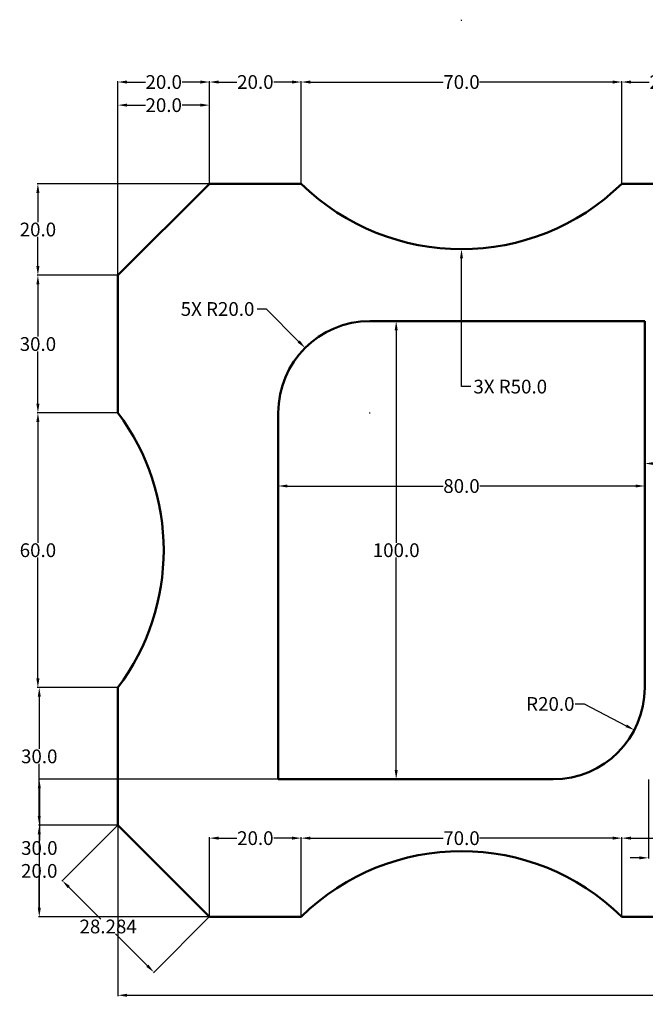
# Model space of a CAD drawing. Units: inches. Extents: x 142 to 482, y 54 to 269.
# Tile 1 of 2: x 142 to 279, y 54 to 269. Entities that reach past the tile are written whole.
import ezdxf

# ---------------------------------------------------------------- set-up
doc = ezdxf.new("R2010")
doc.units = ezdxf.units.IN
doc.header["$MEASUREMENT"] = 0
doc.layers.add('M-DIMS', color=2, linetype='Continuous', lineweight=25)
doc.layers.add('M-OUTL', color=7, linetype='Continuous', lineweight=50)
doc.styles.get("Standard").update_dxf_attribs({"font": 'arial.ttf'})
doc.dimstyles.get("Standard").update_dxf_attribs({"dimtxt": 3, "dimasz": 2, "dimexe": 0.18, "dimexo": 0.0625, "dimgap": 0.09, "dimtad": 0, "dimtih": 1, "dimtoh": 1, "dimdec": 1, "dimzin": 0, "dimdsep": 46, "dimtxsty": 'Standard', "dimcen": 0.09, "dimclrd": 1, "dimclre": 1, "dimadec": 0, "dimazin": 0, "dimtfac": 1, "dimtdec": 1, "dimtofl": 0, "dimtmove": 0, "dimatfit": 3, "dimfxl": 1, "dimtolj": 1, "dimtzin": 0, "dimarcsym": 0})

# ---------------------------------------------------------------- blocks, each defined once
blk = doc.blocks.new('*D1')
at = {"layer": 'Defpoints', "color": 0, "transparency": 16777216}
for p in [(146.28, 183.54), (163.74, 183.54), (163.74, 123.54)]:
    blk.add_point(p, dxfattribs=at)
at = {"layer": 'M-DIMS', "color": 0, "lineweight": -2, "transparency": 16777216}
for p, q in [((163.67, 183.54), (146.1, 183.54)), ((146.28, 181.54), (146.28, 155.16)), ((146.28, 125.54), (146.28, 151.92)), ((163.67, 123.54), (146.1, 123.54))]:
    blk.add_line(p, q, dxfattribs=at)
at = {"layer": 'M-DIMS', "color": 0, "transparency": 16777216}
for points in [[(145.94, 181.54), (146.61, 181.54), (146.28, 183.54)], [(145.94, 125.54), (146.61, 125.54), (146.28, 123.54)]]:
    blk.add_solid(points, dxfattribs=at)
at = {"layer": 'M-DIMS', "color": 0, "transparency": 16777216, "insert": (146.28, 153.54), "char_height": 3, "attachment_point": 5}
blk.add_mtext('\\A1;60.0', dxfattribs=at)
blk = doc.blocks.new('*D2')
at = {"layer": 'Defpoints', "color": 0, "transparency": 16777216}
for p in [(163.74, 93.54), (146.57, 73.54), (183.74, 73.54)]:
    blk.add_point(p, dxfattribs=at)
at = {"layer": 'M-DIMS', "color": 0, "lineweight": -2, "transparency": 16777216}
for p, q in [((163.67, 93.54), (146.39, 93.54)), ((146.57, 91.54), (146.57, 85.16)), ((146.57, 75.54), (146.57, 81.92)), ((183.67, 73.54), (146.39, 73.54))]:
    blk.add_line(p, q, dxfattribs=at)
at = {"layer": 'M-DIMS', "color": 0, "transparency": 16777216}
for points in [[(146.24, 91.54), (146.91, 91.54), (146.57, 93.54)], [(146.24, 75.54), (146.91, 75.54), (146.57, 73.54)]]:
    blk.add_solid(points, dxfattribs=at)
at = {"layer": 'M-DIMS', "color": 0, "transparency": 16777216, "insert": (146.57, 83.54), "char_height": 3, "attachment_point": 5}
blk.add_mtext('\\A1;20.0', dxfattribs=at)
blk = doc.blocks.new('*D3')
at = {"layer": 'Defpoints', "color": 0, "transparency": 16777216}
for p in [(146.57, 123.54), (163.74, 123.54), (163.74, 93.54)]:
    blk.add_point(p, dxfattribs=at)
at = {"layer": 'M-DIMS', "color": 0, "lineweight": -2, "transparency": 16777216}
for p, q in [((163.67, 123.54), (146.39, 123.54)), ((146.57, 121.54), (146.57, 110.16)), ((146.57, 95.54), (146.57, 106.92)), ((163.67, 93.54), (146.39, 93.54))]:
    blk.add_line(p, q, dxfattribs=at)
at = {"layer": 'M-DIMS', "color": 0, "transparency": 16777216}
for points in [[(146.24, 121.54), (146.91, 121.54), (146.57, 123.54)], [(146.24, 95.54), (146.91, 95.54), (146.57, 93.54)]]:
    blk.add_solid(points, dxfattribs=at)
at = {"layer": 'M-DIMS', "color": 0, "transparency": 16777216, "insert": (146.57, 108.54), "char_height": 3, "attachment_point": 5}
blk.add_mtext('\\A1;30.0', dxfattribs=at)
blk = doc.blocks.new('*D4')
at = {"layer": 'Defpoints', "color": 0, "transparency": 16777216}
for p in [(146.28, 213.54), (163.74, 213.54), (163.74, 183.54)]:
    blk.add_point(p, dxfattribs=at)
at = {"layer": 'M-DIMS', "color": 0, "lineweight": -2, "transparency": 16777216}
for p, q in [((163.67, 213.54), (146.1, 213.54)), ((146.28, 211.54), (146.28, 200.16)), ((146.28, 185.54), (146.28, 196.92)), ((163.67, 183.54), (146.1, 183.54))]:
    blk.add_line(p, q, dxfattribs=at)
at = {"layer": 'M-DIMS', "color": 0, "transparency": 16777216}
for points in [[(145.94, 211.54), (146.61, 211.54), (146.28, 213.54)], [(145.94, 185.54), (146.61, 185.54), (146.28, 183.54)]]:
    blk.add_solid(points, dxfattribs=at)
at = {"layer": 'M-DIMS', "color": 0, "transparency": 16777216, "insert": (146.28, 198.54), "char_height": 3, "attachment_point": 5}
blk.add_mtext('\\A1;30.0', dxfattribs=at)
blk = doc.blocks.new('*D5')
at = {"layer": 'Defpoints', "color": 0, "transparency": 16777216}
for p in [(183.74, 233.54), (146.28, 213.54), (163.74, 213.54)]:
    blk.add_point(p, dxfattribs=at)
at = {"layer": 'M-DIMS', "color": 0, "lineweight": -2, "transparency": 16777216}
for p, q in [((183.67, 233.54), (146.1, 233.54)), ((146.28, 231.54), (146.28, 225.16)), ((146.28, 215.54), (146.28, 221.92)), ((163.67, 213.54), (146.1, 213.54))]:
    blk.add_line(p, q, dxfattribs=at)
at = {"layer": 'M-DIMS', "color": 0, "transparency": 16777216}
for points in [[(145.94, 231.54), (146.61, 231.54), (146.28, 233.54)], [(145.94, 215.54), (146.61, 215.54), (146.28, 213.54)]]:
    blk.add_solid(points, dxfattribs=at)
at = {"layer": 'M-DIMS', "color": 0, "transparency": 16777216, "insert": (146.28, 223.54), "char_height": 3, "attachment_point": 5}
blk.add_mtext('\\A1;20.0', dxfattribs=at)
blk = doc.blocks.new('*D6')
at = {"layer": 'Defpoints', "color": 0, "transparency": 16777216}
for p in [(203.74, 255.73), (183.74, 233.54), (203.74, 233.54)]:
    blk.add_point(p, dxfattribs=at)
at = {"layer": 'M-DIMS', "color": 0, "lineweight": -2, "transparency": 16777216}
for p, q in [((183.74, 233.6), (183.74, 255.91)), ((203.74, 233.6), (203.74, 255.91)), ((185.74, 255.73), (189.73, 255.73)), ((201.74, 255.73), (197.74, 255.73))]:
    blk.add_line(p, q, dxfattribs=at)
at = {"layer": 'M-DIMS', "color": 0, "transparency": 16777216}
for points in [[(185.74, 256.06), (185.74, 255.39), (183.74, 255.73)], [(201.74, 256.06), (201.74, 255.39), (203.74, 255.73)]]:
    blk.add_solid(points, dxfattribs=at)
at = {"layer": 'M-DIMS', "color": 0, "transparency": 16777216, "insert": (193.74, 255.73), "char_height": 3, "attachment_point": 5}
blk.add_mtext('\\A1;20.0', dxfattribs=at)
blk = doc.blocks.new('*D7')
at = {"layer": 'Defpoints', "color": 0, "transparency": 16777216}
for p in [(163.74, 255.73), (183.74, 233.54), (163.74, 213.54)]:
    blk.add_point(p, dxfattribs=at)
at = {"layer": 'M-DIMS', "color": 0, "lineweight": -2, "transparency": 16777216}
for p, q in [((163.74, 213.6), (163.74, 255.91)), ((183.74, 233.6), (183.74, 255.91)), ((165.74, 255.73), (169.73, 255.73)), ((181.74, 255.73), (177.74, 255.73))]:
    blk.add_line(p, q, dxfattribs=at)
at = {"layer": 'M-DIMS', "color": 0, "transparency": 16777216}
for points in [[(165.74, 256.06), (165.74, 255.39), (163.74, 255.73)], [(181.74, 256.06), (181.74, 255.39), (183.74, 255.73)]]:
    blk.add_solid(points, dxfattribs=at)
at = {"layer": 'M-DIMS', "color": 0, "transparency": 16777216, "insert": (173.74, 255.73), "char_height": 3, "attachment_point": 5}
blk.add_mtext('\\A1;20.0', dxfattribs=at)
blk = doc.blocks.new('*D8')
at = {"layer": 'Defpoints', "color": 0, "transparency": 16777216}
for p in [(273.74, 255.73), (203.74, 233.54), (273.74, 233.54)]:
    blk.add_point(p, dxfattribs=at)
at = {"layer": 'M-DIMS', "color": 0, "lineweight": -2, "transparency": 16777216}
for p, q in [((203.74, 233.6), (203.74, 255.91)), ((273.74, 233.6), (273.74, 255.91)), ((205.74, 255.73), (234.77, 255.73)), ((271.74, 255.73), (242.7, 255.73))]:
    blk.add_line(p, q, dxfattribs=at)
at = {"layer": 'M-DIMS', "color": 0, "transparency": 16777216}
for points in [[(205.74, 256.06), (205.74, 255.39), (203.74, 255.73)], [(271.74, 256.06), (271.74, 255.39), (273.74, 255.73)]]:
    blk.add_solid(points, dxfattribs=at)
at = {"layer": 'M-DIMS', "color": 0, "transparency": 16777216, "insert": (238.74, 255.73), "char_height": 3, "attachment_point": 5}
blk.add_mtext('\\A1;70.0', dxfattribs=at)
blk = doc.blocks.new('*D9')
at = {"layer": 'Defpoints', "color": 0, "transparency": 16777216}
for p in [(293.74, 255.73), (273.74, 233.54), (293.74, 233.54)]:
    blk.add_point(p, dxfattribs=at)
at = {"layer": 'M-DIMS', "color": 0, "lineweight": -2, "transparency": 16777216}
for p, q in [((273.74, 233.6), (273.74, 255.91)), ((293.74, 233.6), (293.74, 255.91)), ((275.74, 255.73), (279.73, 255.73)), ((291.74, 255.73), (287.74, 255.73))]:
    blk.add_line(p, q, dxfattribs=at)
at = {"layer": 'M-DIMS', "color": 0, "transparency": 16777216}
for points in [[(275.74, 256.06), (275.74, 255.39), (273.74, 255.73)], [(291.74, 256.06), (291.74, 255.39), (293.74, 255.73)]]:
    blk.add_solid(points, dxfattribs=at)
at = {"layer": 'M-DIMS', "color": 0, "transparency": 16777216, "insert": (283.74, 255.73), "char_height": 3, "attachment_point": 5}
blk.add_mtext('\\A1;20.0', dxfattribs=at)
blk = doc.blocks.new('*D22')
at = {"layer": 'Defpoints', "color": 0, "transparency": 16777216}
for p in [(258.74, 123.54), (276.47, 114.29)]:
    blk.add_point(p, dxfattribs=at)
at = {"layer": 'M-DIMS', "color": 0, "lineweight": -2, "transparency": 16777216}
for p, q in [((263.55, 119.98), (265.55, 119.98)), ((265.55, 119.98), (274.69, 115.21))]:
    blk.add_line(p, q, dxfattribs=at)
at = {"layer": 'M-DIMS', "color": 0, "transparency": 16777216}
blk.add_solid([(274.85, 115.51), (274.54, 114.92), (276.47, 114.29)], dxfattribs=at)
at = {"layer": 'M-DIMS', "color": 0, "transparency": 16777216, "insert": (258.13, 119.98), "char_height": 3, "attachment_point": 5}
blk.add_mtext('\\A1;R20.0', dxfattribs=at)
blk = doc.blocks.new('*D23')
at = {"layer": 'Defpoints', "color": 0, "transparency": 16777216}
for p in [(248.74, 203.54), (224.48, 103.54), (228.74, 103.54)]:
    blk.add_point(p, dxfattribs=at)
at = {"layer": 'M-DIMS', "color": 0, "lineweight": -2, "transparency": 16777216}
for p, q in [((248.67, 203.54), (224.3, 203.54)), ((224.48, 201.54), (224.48, 155.16)), ((224.48, 105.54), (224.48, 151.92)), ((228.67, 103.54), (224.3, 103.54))]:
    blk.add_line(p, q, dxfattribs=at)
at = {"layer": 'M-DIMS', "color": 0, "transparency": 16777216}
for points in [[(224.15, 201.54), (224.81, 201.54), (224.48, 203.54)], [(224.15, 105.54), (224.81, 105.54), (224.48, 103.54)]]:
    blk.add_solid(points, dxfattribs=at)
at = {"layer": 'M-DIMS', "color": 0, "transparency": 16777216, "insert": (224.48, 153.54), "char_height": 3, "attachment_point": 5}
blk.add_mtext('\\A1;100.0', dxfattribs=at)
blk = doc.blocks.new('*D24')
at = {"layer": 'Defpoints', "color": 0, "transparency": 16777216}
for p in [(198.74, 183.54), (278.74, 183.54), (278.74, 167.55)]:
    blk.add_point(p, dxfattribs=at)
at = {"layer": 'M-DIMS', "color": 0, "lineweight": -2, "transparency": 16777216}
for p, q in [((198.74, 183.48), (198.74, 167.37)), ((278.74, 183.48), (278.74, 167.37)), ((200.74, 167.55), (234.75, 167.55)), ((276.74, 167.55), (242.72, 167.55))]:
    blk.add_line(p, q, dxfattribs=at)
at = {"layer": 'M-DIMS', "color": 0, "transparency": 16777216}
for points in [[(200.74, 167.88), (200.74, 167.22), (198.74, 167.55)], [(276.74, 167.88), (276.74, 167.22), (278.74, 167.55)]]:
    blk.add_solid(points, dxfattribs=at)
at = {"layer": 'M-DIMS', "color": 0, "transparency": 16777216, "insert": (238.74, 167.55), "char_height": 3, "attachment_point": 5}
blk.add_mtext('\\A1;80.0', dxfattribs=at)
blk = doc.blocks.new('*D26')
at = {"layer": 'Defpoints', "color": 0, "transparency": 16777216}
for p in [(278.74, 183.54), (313.74, 183.54), (313.74, 172.46)]:
    blk.add_point(p, dxfattribs=at)
at = {"layer": 'M-DIMS', "color": 0, "lineweight": -2, "transparency": 16777216}
for p, q in [((278.74, 183.48), (278.74, 172.28)), ((313.74, 183.48), (313.74, 172.28)), ((280.74, 172.46), (292.26, 172.46)), ((311.74, 172.46), (300.22, 172.46))]:
    blk.add_line(p, q, dxfattribs=at)
at = {"layer": 'M-DIMS', "color": 0, "transparency": 16777216}
for points in [[(280.74, 172.79), (280.74, 172.13), (278.74, 172.46)], [(311.74, 172.79), (311.74, 172.13), (313.74, 172.46)]]:
    blk.add_solid(points, dxfattribs=at)
at = {"layer": 'M-DIMS', "color": 0, "transparency": 16777216, "insert": (296.24, 172.46), "char_height": 3, "attachment_point": 5}
blk.add_mtext('\\A1;35.0', dxfattribs=at)
blk = doc.blocks.new('*D27')
at = {"layer": 'Defpoints', "color": 0, "transparency": 16777216}
for p in [(450.34, 141.94), (163.74, 93.54), (450.34, 56.39)]:
    blk.add_point(p, dxfattribs=at)
at = {"layer": 'M-DIMS', "color": 1, "lineweight": -2, "transparency": 16777216}
for p, q in [((450.34, 141.88), (450.34, 56.21)), ((163.74, 93.48), (163.74, 56.21)), ((165.74, 56.39), (301.86, 56.39)), ((448.34, 56.39), (312.21, 56.39))]:
    blk.add_line(p, q, dxfattribs=at)
at = {"layer": 'M-DIMS', "color": 1, "transparency": 16777216}
for points in [[(165.74, 56.72), (165.74, 56.06), (163.74, 56.39)], [(448.34, 56.72), (448.34, 56.06), (450.34, 56.39)]]:
    blk.add_solid(points, dxfattribs=at)
at = {"layer": 'M-DIMS', "color": 0, "transparency": 16777216, "insert": (307.04, 56.39), "char_height": 3, "attachment_point": 5}
blk.add_mtext('\\A1;286.6', dxfattribs=at)
blk = doc.blocks.new('*D29')
at = {"layer": 'Defpoints', "color": 0, "transparency": 16777216}
for p in [(198.74, 103.54), (146.59, 73.54), (183.74, 73.54)]:
    blk.add_point(p, dxfattribs=at)
at = {"layer": 'M-DIMS', "color": 1, "lineweight": -2, "transparency": 16777216}
for p, q in [((198.67, 103.54), (146.41, 103.54)), ((146.59, 101.54), (146.59, 90.16)), ((146.59, 75.54), (146.59, 86.92)), ((183.67, 73.54), (146.41, 73.54))]:
    blk.add_line(p, q, dxfattribs=at)
at = {"layer": 'M-DIMS', "color": 1, "transparency": 16777216}
for points in [[(146.25, 101.54), (146.92, 101.54), (146.59, 103.54)], [(146.25, 75.54), (146.92, 75.54), (146.59, 73.54)]]:
    blk.add_solid(points, dxfattribs=at)
at = {"layer": 'M-DIMS', "color": 0, "transparency": 16777216, "insert": (146.59, 88.54), "char_height": 3, "attachment_point": 5}
blk.add_mtext('\\A1;30.0', dxfattribs=at)
blk = doc.blocks.new('*D36')
at = {"layer": 'Defpoints', "color": 0, "transparency": 16777216}
for p in [(279.57, 103.54), (294.34, 103.54), (279.57, 86.39)]:
    blk.add_point(p, dxfattribs=at)
at = {"layer": 'M-DIMS', "color": 1, "lineweight": -2, "transparency": 16777216}
for p, q in [((279.57, 103.48), (279.57, 86.21)), ((294.34, 103.48), (294.34, 86.21)), ((277.57, 86.39), (275.57, 86.39)), ((296.34, 86.39), (298.34, 86.39))]:
    blk.add_line(p, q, dxfattribs=at)
at = {"layer": 'M-DIMS', "color": 1, "transparency": 16777216}
for points in [[(277.57, 86.72), (277.57, 86.06), (279.57, 86.39)], [(296.34, 86.72), (296.34, 86.06), (294.34, 86.39)]]:
    blk.add_solid(points, dxfattribs=at)
at = {"layer": 'M-DIMS', "color": 0, "transparency": 16777216, "insert": (286.95, 86.39), "char_height": 3, "attachment_point": 5}
blk.add_mtext('\\A1;14.776', dxfattribs=at)
blk = doc.blocks.new('*D37')
at = {"layer": 'Defpoints', "color": 0, "transparency": 16777216}
for p in [(284.73, 90.69), (273.74, 73.54), (284.73, 73.54)]:
    blk.add_point(p, dxfattribs=at)
at = {"layer": 'M-DIMS', "color": 1, "lineweight": -2, "transparency": 16777216}
for p, q in [((273.74, 73.6), (273.74, 90.87)), ((275.74, 90.69), (282.73, 90.69)), ((284.73, 73.6), (284.73, 90.87)), ((284.73, 90.69), (286.73, 90.69))]:
    blk.add_line(p, q, dxfattribs=at)
at = {"layer": 'M-DIMS', "color": 1, "transparency": 16777216}
for points in [[(275.74, 91.02), (275.74, 90.36), (273.74, 90.69)], [(282.73, 91.02), (282.73, 90.36), (284.73, 90.69)]]:
    blk.add_solid(points, dxfattribs=at)
at = {"layer": 'M-DIMS', "color": 0, "transparency": 16777216, "insert": (292.91, 90.69), "char_height": 3, "attachment_point": 5}
blk.add_mtext('\\A1;10.999', dxfattribs=at)
blk = doc.blocks.new('*D41')
at = {"layer": 'Defpoints', "color": 0, "transparency": 16777216}
for p in [(183.74, 250.69), (183.74, 233.54), (163.74, 213.54)]:
    blk.add_point(p, dxfattribs=at)
at = {"layer": 'M-DIMS', "color": 1, "lineweight": -2, "transparency": 16777216}
for p, q in [((163.74, 213.6), (163.74, 250.87)), ((165.74, 250.69), (169.73, 250.69)), ((181.74, 250.69), (177.74, 250.69)), ((183.74, 233.6), (183.74, 250.87))]:
    blk.add_line(p, q, dxfattribs=at)
at = {"layer": 'M-DIMS', "color": 1, "transparency": 16777216}
for points in [[(165.74, 251.02), (165.74, 250.36), (163.74, 250.69)], [(181.74, 251.02), (181.74, 250.36), (183.74, 250.69)]]:
    blk.add_solid(points, dxfattribs=at)
at = {"layer": 'M-DIMS', "color": 0, "transparency": 16777216, "insert": (173.74, 250.69), "char_height": 3, "attachment_point": 5}
blk.add_mtext('\\A1;20.0', dxfattribs=at)
blk = doc.blocks.new('*D42')
at = {"layer": 'Defpoints', "color": 0, "transparency": 16777216}
for p in [(203.74, 90.69), (183.74, 73.54), (203.74, 73.54)]:
    blk.add_point(p, dxfattribs=at)
at = {"layer": 'M-DIMS', "color": 1, "lineweight": -2, "transparency": 16777216}
for p, q in [((183.74, 73.6), (183.74, 90.87)), ((185.74, 90.69), (189.73, 90.69)), ((201.74, 90.69), (197.74, 90.69)), ((203.74, 73.6), (203.74, 90.87))]:
    blk.add_line(p, q, dxfattribs=at)
at = {"layer": 'M-DIMS', "color": 1, "transparency": 16777216}
for points in [[(185.74, 91.02), (185.74, 90.36), (183.74, 90.69)], [(201.74, 91.02), (201.74, 90.36), (203.74, 90.69)]]:
    blk.add_solid(points, dxfattribs=at)
at = {"layer": 'M-DIMS', "color": 0, "transparency": 16777216, "insert": (193.74, 90.69), "char_height": 3, "attachment_point": 5}
blk.add_mtext('\\A1;20.0', dxfattribs=at)
blk = doc.blocks.new('*D43')
at = {"layer": 'Defpoints', "color": 0, "transparency": 16777216}
for p in [(273.74, 90.69), (203.74, 73.54), (273.74, 73.54)]:
    blk.add_point(p, dxfattribs=at)
at = {"layer": 'M-DIMS', "color": 1, "lineweight": -2, "transparency": 16777216}
for p, q in [((203.74, 73.6), (203.74, 90.87)), ((205.74, 90.69), (234.77, 90.69)), ((271.74, 90.69), (242.7, 90.69)), ((273.74, 73.6), (273.74, 90.87))]:
    blk.add_line(p, q, dxfattribs=at)
at = {"layer": 'M-DIMS', "color": 1, "transparency": 16777216}
for points in [[(205.74, 91.02), (205.74, 90.36), (203.74, 90.69)], [(271.74, 91.02), (271.74, 90.36), (273.74, 90.69)]]:
    blk.add_solid(points, dxfattribs=at)
at = {"layer": 'M-DIMS', "color": 0, "transparency": 16777216, "insert": (238.74, 90.69), "char_height": 3, "attachment_point": 5}
blk.add_mtext('\\A1;70.0', dxfattribs=at)
blk = doc.blocks.new('*D45')
at = {"layer": 'Defpoints', "color": 0, "transparency": 16777216}
for p in [(163.74, 93.54), (151.61, 81.41), (183.74, 73.54)]:
    blk.add_point(p, dxfattribs=at)
at = {"layer": 'M-DIMS', "color": 1, "lineweight": -2, "transparency": 16777216}
for p, q in [((163.69, 93.49), (151.48, 81.28)), ((153.02, 80), (159.99, 73.03)), ((183.69, 73.49), (171.48, 61.28)), ((170.19, 62.83), (163.23, 69.79))]:
    blk.add_line(p, q, dxfattribs=at)
at = {"layer": 'M-DIMS', "color": 1, "transparency": 16777216}
for points in [[(153.26, 80.23), (152.79, 79.76), (151.61, 81.41)], [(170.43, 63.06), (169.96, 62.59), (171.61, 61.41)]]:
    blk.add_solid(points, dxfattribs=at)
at = {"layer": 'M-DIMS', "color": 0, "transparency": 16777216, "insert": (161.61, 71.41), "char_height": 3, "attachment_point": 5}
blk.add_mtext('\\A1;28.284', dxfattribs=at)
blk = doc.blocks.new('*D47')
at = {"layer": 'Defpoints', "color": 0, "transparency": 16777216}
for p in [(204.61, 197.69), (218.74, 183.54)]:
    blk.add_point(p, dxfattribs=at)
at = {"layer": 'M-DIMS', "color": 1, "lineweight": -2, "transparency": 16777216}
for p, q in [((194.13, 206.19), (196.13, 206.19)), ((196.13, 206.19), (203.19, 199.11)), ((218.65, 183.54), (218.83, 183.54)), ((218.74, 183.45), (218.74, 183.63))]:
    blk.add_line(p, q, dxfattribs=at)
at = {"layer": 'M-DIMS', "color": 1, "transparency": 16777216}
blk.add_solid([(203.43, 199.34), (202.96, 198.87), (204.61, 197.69)], dxfattribs=at)
at = {"layer": 'M-DIMS', "color": 0, "transparency": 16777216, "insert": (185.49, 206.19), "char_height": 3, "attachment_point": 5}
blk.add_mtext('\\A1;5X R20.0', dxfattribs=at)
blk = doc.blocks.new('*D50')
at = {"layer": 'Defpoints', "color": 0, "transparency": 16777216}
for p in [(238.74, 269.25), (238.74, 219.25)]:
    blk.add_point(p, dxfattribs=at)
at = {"layer": 'M-DIMS', "color": 1, "lineweight": -2, "transparency": 16777216}
for p, q in [((238.65, 269.25), (238.83, 269.25)), ((238.74, 269.16), (238.74, 269.34)), ((238.74, 189.25), (238.74, 217.25)), ((240.74, 189.25), (238.74, 189.25))]:
    blk.add_line(p, q, dxfattribs=at)
at = {"layer": 'M-DIMS', "color": 1, "transparency": 16777216}
blk.add_solid([(239.07, 217.25), (238.41, 217.25), (238.74, 219.25)], dxfattribs=at)
at = {"layer": 'M-DIMS', "color": 0, "transparency": 16777216, "insert": (249.38, 189.25), "char_height": 3, "attachment_point": 5}
blk.add_mtext('\\A1;3X R50.0', dxfattribs=at)

msp = doc.modelspace()

# ---------------------------------------------------------------- linework, layer by layer
at = {"layer": 'M-OUTL'}
for p, q in [((163.7359, 213.539), (183.7359, 233.539)), ((183.7359, 233.539), (203.7359, 233.539)), ((273.7359, 233.539), (293.7359, 233.539)), ((163.7359, 183.539), (163.7359, 213.539)), ((278.7359, 203.539), (218.7359, 203.539)), ((278.7359, 183.539), (278.7359, 203.539)), ((198.7359, 183.539), (198.7359, 103.539)), ((278.7359, 123.539), (278.7359, 183.539)), ((163.7359, 93.539), (163.7359, 123.539)), ((198.7359, 103.539), (258.7359, 103.539)), ((163.7359, 93.539), (183.7359, 73.539)), ((183.7359, 73.539), (203.7359, 73.539)), ((273.7359, 73.539), (284.7346, 73.539))]:
    msp.add_line(p, q, dxfattribs=at)
for centre, radius, start, end in [((238.7359, 269.2461), 50, 225.572996, 314.427004), ((218.7359, 183.539), 20, 90, 180), ((123.7359, 153.539), 50, 323.130102, 36.869898), ((258.7359, 123.539), 20, 270, 0), ((238.7359, 37.8318), 50, 45.572996, 134.427004)]:
    msp.add_arc(centre, radius, start, end, dxfattribs=at)

# ---------------------------------------------------------------- dimensions: what is measured, and where the dimension line sits
at = {"layer": 'M-DIMS'}
for center, mpoint, text, picture, middle in [((238.7359, 269.2461), (238.74, 219.2461), '3X <>', '*D50', (249.3813, 189.2461)), ((218.7359, 183.539), (204.6063, 197.6937), '5X <>', '*D47', (185.4888, 206.1865))]:
    dim = msp.add_radius_dim(center=center, mpoint=mpoint, text=text, dimstyle='Standard', override={"dimdec": 1, "dimlfac": 1, "dimrnd": 0, "dimzin": 0, "dimdsep": 46, "dimlunit": 2}, dxfattribs=at)
    dim.commit()
    dim.dimension.update_dxf_attribs({"geometry": picture, "text_midpoint": middle, "dimtype": 164})
for base, p1, p2, override, picture, middle in [((163.7359, 255.7265), (183.7359, 233.539), (163.7359, 213.539), {"dimclrd": 0, "dimclre": 0, "dimclrt": 0}, '*D7', (173.7359, 255.7265)), ((203.7359, 255.7265), (183.7359, 233.539), (203.7359, 233.539), {"dimclrd": 0, "dimclre": 0, "dimclrt": 0}, '*D6', (193.7359, 255.7265)), ((273.7359, 255.7265), (203.7359, 233.539), (273.7359, 233.539), {"dimclrd": 0, "dimclre": 0, "dimclrt": 0}, '*D8', (238.7359, 255.7265)), ((293.7359, 255.7265), (273.7359, 233.539), (293.7359, 233.539), {"dimclrd": 0, "dimclre": 0, "dimclrt": 0}, '*D9', (283.7359, 255.7265)), ((183.7359, 250.689), (163.7359, 213.539), (183.7359, 233.539), {"dimdec": 1, "dimlfac": 1, "dimrnd": 0, "dimzin": 0, "dimdsep": 46, "dimlunit": 2}, '*D41', (173.7359, 250.689)), ((278.7359, 167.5509), (198.7359, 183.539), (278.7359, 183.539), {"dimclrd": 0, "dimclre": 0, "dimclrt": 0}, '*D24', (238.7359, 167.5509)), ((313.7359, 172.4595), (278.7359, 183.539), (313.7359, 183.539), {"dimclrd": 0, "dimclre": 0, "dimclrt": 0}, '*D26', (296.2359, 172.4595)), ((450.3359, 56.389), (163.7359, 93.539), (450.3359, 141.939), {"dimdec": 1, "dimlfac": 1, "dimrnd": 0, "dimzin": 0, "dimdsep": 46, "dimlunit": 2}, '*D27', (307.0359, 56.389)), ((273.7359, 90.689), (203.7359, 73.539), (273.7359, 73.539), {"dimdec": 1, "dimlfac": 1, "dimrnd": 0, "dimzin": 0, "dimdsep": 46, "dimlunit": 2}, '*D43', (238.7359, 90.689))]:
    dim = msp.add_linear_dim(base=base, p1=p1, p2=p2, dimstyle='Standard', override=override, dxfattribs=at)
    dim.commit()
    dim.dimension.update_dxf_attribs({"geometry": picture, "text_midpoint": middle})
for base, p1, p2, angle, override, picture, middle in [((146.2778, 213.539), (183.7359, 233.539), (163.7359, 213.539), 90, {"dimclrd": 0, "dimclre": 0, "dimclrt": 0}, '*D5', (146.2778, 223.539)), ((146.2778, 213.539), (163.7359, 183.539), (163.7359, 213.539), 90, {"dimclrd": 0, "dimclre": 0, "dimclrt": 0}, '*D4', (146.2778, 198.539)), ((224.479, 103.539), (248.7359, 203.539), (228.7359, 103.539), 90, {"dimclrd": 0, "dimclre": 0, "dimclrt": 0}, '*D23', (224.479, 153.539)), ((146.5718, 123.539), (163.7359, 93.539), (163.7359, 123.539), 90, {"dimclrd": 0, "dimclre": 0, "dimclrt": 0}, '*D3', (146.5718, 108.539)), ((146.5859, 73.539), (198.7359, 103.539), (183.7359, 73.539), 90, {"dimdec": 1, "dimlfac": 1, "dimrnd": 0, "dimzin": 0, "dimdsep": 46, "dimlunit": 2}, '*D29', (146.5859, 88.539)), ((279.566, 86.389), (294.3424, 103.539), (279.566, 103.539), 180, {"dimdec": 3, "dimlfac": 1, "dimrnd": 0, "dimzin": 0, "dimdsep": 46, "dimlunit": 2}, '*D36', (286.9542, 86.389)), ((146.5718, 73.539), (163.7359, 93.539), (183.7359, 73.539), 90, {"dimclrd": 0, "dimclre": 0, "dimclrt": 0}, '*D2', (146.5718, 83.539)), ((151.609, 81.4121), (183.7359, 73.539), (163.7359, 93.539), 135, {"dimdec": 3, "dimlfac": 1, "dimrnd": 0, "dimzin": 0, "dimdsep": 46, "dimlunit": 2}, '*D45', (161.609, 71.4121)), ((203.7359, 90.689), (183.7359, 73.539), (203.7359, 73.539), 0, {"dimdec": 1, "dimlfac": 1, "dimrnd": 0, "dimzin": 0, "dimdsep": 46, "dimlunit": 2}, '*D42', (193.7359, 90.689)), ((284.7346, 90.689), (273.7359, 73.539), (284.7346, 73.539), 0, {"dimdec": 3, "dimlfac": 1, "dimrnd": 0, "dimzin": 0, "dimdsep": 46, "dimlunit": 2}, '*D37', (292.9137, 90.689))]:
    dim = msp.add_linear_dim(base=base, p1=p1, p2=p2, angle=angle, dimstyle='Standard', override=override, dxfattribs=at)
    dim.commit()
    dim.dimension.update_dxf_attribs({"geometry": picture, "text_midpoint": middle})
dim = msp.add_linear_dim(base=(146.2778, 183.539), p1=(163.7359, 123.539), p2=(163.7359, 183.539), angle=90, dimstyle='Standard', override={"dimclrd": 0, "dimclre": 0, "dimclrt": 0}, dxfattribs=at)
dim.commit()
dim.dimension.update_dxf_attribs({"geometry": '*D1', "text_midpoint": (146.2778, 153.539), "dimtype": 160})
dim = msp.add_radius_dim(center=(258.7359, 123.539), mpoint=(276.4664, 114.2855), dimstyle='Standard', override={"dimclrd": 0, "dimclre": 0, "dimclrt": 0}, dxfattribs=at)
dim.commit()
dim.dimension.update_dxf_attribs({"geometry": '*D22', "text_midpoint": (258.1349, 119.9818), "dimtype": 164})

doc.saveas('drawing.dxf')
